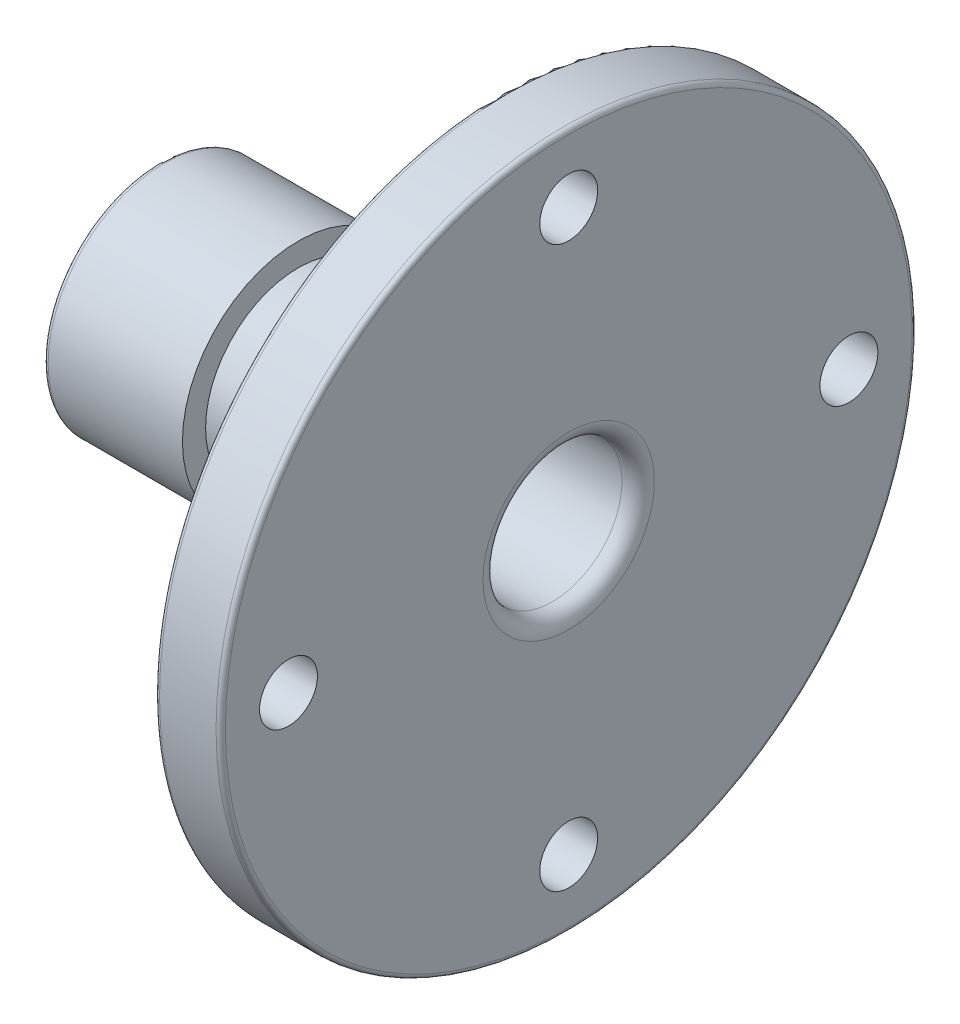
ISO-10303-21;
HEADER;
FILE_DESCRIPTION(('STEP AP214'),'2;1');
FILE_NAME('part.step','',(''),(''),'','','');
FILE_SCHEMA(('AUTOMOTIVE_DESIGN { 1 0 10303 214 1 1 1 1 }'));
ENDSEC;
DATA;
#1=APPLICATION_CONTEXT('core data for automotive mechanical design processes');
#2=APPLICATION_PROTOCOL_DEFINITION('international standard','automotive_design',2000,#1);
#3=PRODUCT_CONTEXT('',#1,'mechanical');
#4=PRODUCT('Part','Part','',(#3));
#5=PRODUCT_RELATED_PRODUCT_CATEGORY('part','',(#4));
#6=PRODUCT_DEFINITION_FORMATION('','',#4);
#7=PRODUCT_DEFINITION_CONTEXT('part definition',#1,'design');
#8=PRODUCT_DEFINITION('design','',#6,#7);
#9=PRODUCT_DEFINITION_SHAPE('','',#8);
#10=(LENGTH_UNIT() NAMED_UNIT(*) SI_UNIT(.MILLI.,.METRE.));
#11=(NAMED_UNIT(*) PLANE_ANGLE_UNIT() SI_UNIT($,.RADIAN.));
#12=(NAMED_UNIT(*) SI_UNIT($,.STERADIAN.) SOLID_ANGLE_UNIT());
#13=UNCERTAINTY_MEASURE_WITH_UNIT(LENGTH_MEASURE(1.E-05),#10,'distance_accuracy_value','');
#14=(GEOMETRIC_REPRESENTATION_CONTEXT(3) GLOBAL_UNCERTAINTY_ASSIGNED_CONTEXT((#13)) GLOBAL_UNIT_ASSIGNED_CONTEXT((#10,
#11,#12)) REPRESENTATION_CONTEXT('',''));
#15=CARTESIAN_POINT('',(0.,0.,0.));
#16=DIRECTION('',(0.,0.,1.));
#17=DIRECTION('',(1.,0.,0.));
#18=AXIS2_PLACEMENT_3D('',#15,#16,#17);
#19=CARTESIAN_POINT('',(0.,20.,0.));
#20=DIRECTION('',(1.,0.,0.));
#21=DIRECTION('',(0.,0.,-1.));
#22=AXIS2_PLACEMENT_3D('',#19,#20,#21);
#23=PLANE('',#22);
#24=CARTESIAN_POINT('',(0.,0.,0.));
#25=DIRECTION('',(1.,0.,0.));
#26=DIRECTION('',(0.,0.,-1.));
#27=AXIS2_PLACEMENT_3D('',#24,#25,#26);
#28=CIRCLE('',#27,24.);
#29=CARTESIAN_POINT('',(0.,0.,-24.));
#30=VERTEX_POINT('',#29);
#31=EDGE_CURVE('E42',#30,#30,#28,.F.);
#32=ORIENTED_EDGE('',*,*,#31,.T.);
#33=EDGE_LOOP('',(#32));
#34=FACE_BOUND('',#33,.T.);
#35=CARTESIAN_POINT('',(0.,0.,0.));
#36=DIRECTION('',(-1.,0.,0.));
#37=DIRECTION('',(0.,0.,1.));
#38=AXIS2_PLACEMENT_3D('',#35,#36,#37);
#39=CIRCLE('',#38,20.);
#40=CARTESIAN_POINT('',(0.,0.,20.));
#41=VERTEX_POINT('',#40);
#42=EDGE_CURVE('E78',#41,#41,#39,.T.);
#43=ORIENTED_EDGE('',*,*,#42,.F.);
#44=EDGE_LOOP('',(#43));
#45=FACE_BOUND('',#44,.T.);
#46=ADVANCED_FACE('F40',(#34,#45),#23,.F.);
#47=CARTESIAN_POINT('',(-1000.,0.,0.));
#48=DIRECTION('',(-1.,0.,0.));
#49=DIRECTION('',(0.,0.,1.));
#50=AXIS2_PLACEMENT_3D('',#47,#48,#49);
#51=CYLINDRICAL_SURFACE('',#50,25.);
#52=CARTESIAN_POINT('',(0.99999999999989,0.,0.));
#53=DIRECTION('',(1.,0.,0.));
#54=DIRECTION('',(0.,0.,-1.));
#55=AXIS2_PLACEMENT_3D('',#52,#53,#54);
#56=CIRCLE('',#55,25.);
#57=CARTESIAN_POINT('',(0.99999999999989,0.,-25.));
#58=VERTEX_POINT('',#57);
#59=EDGE_CURVE('E10',#58,#58,#56,.T.);
#60=ORIENTED_EDGE('',*,*,#59,.T.);
#61=EDGE_LOOP('',(#60));
#62=FACE_BOUND('',#61,.T.);
#63=CARTESIAN_POINT('',(30.,0.,0.));
#64=DIRECTION('',(-1.,0.,0.));
#65=DIRECTION('',(0.,0.,1.));
#66=AXIS2_PLACEMENT_3D('',#63,#64,#65);
#67=CIRCLE('',#66,25.);
#68=CARTESIAN_POINT('',(30.,0.,25.));
#69=VERTEX_POINT('',#68);
#70=EDGE_CURVE('E73',#69,#69,#67,.T.);
#71=ORIENTED_EDGE('',*,*,#70,.T.);
#72=EDGE_LOOP('',(#71));
#73=FACE_BOUND('',#72,.T.);
#74=ADVANCED_FACE('F156',(#62,#73),#51,.T.);
#75=CARTESIAN_POINT('',(30.,25.,0.));
#76=DIRECTION('',(-1.,0.,0.));
#77=DIRECTION('',(0.,0.,1.));
#78=AXIS2_PLACEMENT_3D('',#75,#76,#77);
#79=PLANE('',#78);
#80=ORIENTED_EDGE('',*,*,#70,.F.);
#81=EDGE_LOOP('',(#80));
#82=FACE_BOUND('',#81,.T.);
#83=CARTESIAN_POINT('',(30.,0.,0.));
#84=DIRECTION('',(-1.,0.,0.));
#85=DIRECTION('',(0.,0.,1.));
#86=AXIS2_PLACEMENT_3D('',#83,#84,#85);
#87=CIRCLE('',#86,20.);
#88=CARTESIAN_POINT('',(30.,0.,20.));
#89=VERTEX_POINT('',#88);
#90=EDGE_CURVE('E95',#89,#89,#87,.T.);
#91=ORIENTED_EDGE('',*,*,#90,.T.);
#92=EDGE_LOOP('',(#91));
#93=FACE_BOUND('',#92,.T.);
#94=ADVANCED_FACE('F165',(#82,#93),#79,.F.);
#95=CARTESIAN_POINT('',(-1000.,0.,0.));
#96=DIRECTION('',(-1.,0.,0.));
#97=DIRECTION('',(0.,0.,1.));
#98=AXIS2_PLACEMENT_3D('',#95,#96,#97);
#99=CYLINDRICAL_SURFACE('',#98,20.);
#100=CARTESIAN_POINT('',(73.1999999999999,0.,0.));
#101=DIRECTION('',(1.,0.,0.));
#102=DIRECTION('',(0.,0.,-1.));
#103=AXIS2_PLACEMENT_3D('',#100,#101,#102);
#104=CIRCLE('',#103,20.);
#105=CARTESIAN_POINT('',(73.1999999999999,0.,-20.));
#106=VERTEX_POINT('',#105);
#107=EDGE_CURVE('E48',#106,#106,#104,.F.);
#108=ORIENTED_EDGE('',*,*,#107,.T.);
#109=EDGE_LOOP('',(#108));
#110=FACE_BOUND('',#109,.T.);
#111=ORIENTED_EDGE('',*,*,#90,.F.);
#112=EDGE_LOOP('',(#111));
#113=FACE_BOUND('',#112,.T.);
#114=ADVANCED_FACE('F121',(#110,#113),#99,.T.);
#115=CARTESIAN_POINT('',(74.2,20.,0.));
#116=DIRECTION('',(1.,0.,0.));
#117=DIRECTION('',(0.,0.,-1.));
#118=AXIS2_PLACEMENT_3D('',#115,#116,#117);
#119=PLANE('',#118);
#120=CARTESIAN_POINT('',(74.2,0.,0.));
#121=DIRECTION('',(1.,0.,0.));
#122=DIRECTION('',(0.,0.,-1.));
#123=AXIS2_PLACEMENT_3D('',#120,#121,#122);
#124=CIRCLE('',#123,74.148420880377);
#125=CARTESIAN_POINT('',(74.2,0.,-74.148420880377));
#126=VERTEX_POINT('',#125);
#127=EDGE_CURVE('E55',#126,#126,#124,.F.);
#128=ORIENTED_EDGE('',*,*,#127,.T.);
#129=EDGE_LOOP('',(#128));
#130=FACE_BOUND('',#129,.T.);
#131=CARTESIAN_POINT('',(74.2,0.,0.));
#132=DIRECTION('',(1.,0.,0.));
#133=DIRECTION('',(0.,0.,-1.));
#134=AXIS2_PLACEMENT_3D('',#131,#132,#133);
#135=CIRCLE('',#134,21.);
#136=CARTESIAN_POINT('',(74.2,0.,-21.));
#137=VERTEX_POINT('',#136);
#138=EDGE_CURVE('E60',#137,#137,#135,.T.);
#139=ORIENTED_EDGE('',*,*,#138,.T.);
#140=EDGE_LOOP('',(#139));
#141=FACE_BOUND('',#140,.T.);
#142=CARTESIAN_POINT('',(74.2,60.5,0.));
#143=DIRECTION('',(-1.,0.,0.));
#144=DIRECTION('',(0.,0.,1.));
#145=AXIS2_PLACEMENT_3D('',#142,#143,#144);
#146=CIRCLE('',#145,6.25);
#147=CARTESIAN_POINT('',(74.2,60.5,6.25));
#148=VERTEX_POINT('',#147);
#149=EDGE_CURVE('E90',#148,#148,#146,.T.);
#150=ORIENTED_EDGE('',*,*,#149,.F.);
#151=EDGE_LOOP('',(#150));
#152=FACE_BOUND('',#151,.T.);
#153=CARTESIAN_POINT('',(74.2,0.,-60.5));
#154=DIRECTION('',(-1.,0.,0.));
#155=DIRECTION('',(0.,0.,1.));
#156=AXIS2_PLACEMENT_3D('',#153,#154,#155);
#157=CIRCLE('',#156,6.25);
#158=CARTESIAN_POINT('',(74.2,0.,-54.25));
#159=VERTEX_POINT('',#158);
#160=EDGE_CURVE('E108',#159,#159,#157,.T.);
#161=ORIENTED_EDGE('',*,*,#160,.F.);
#162=EDGE_LOOP('',(#161));
#163=FACE_BOUND('',#162,.T.);
#164=CARTESIAN_POINT('',(74.2,-60.5,0.));
#165=DIRECTION('',(-1.,0.,0.));
#166=DIRECTION('',(0.,0.,-1.));
#167=AXIS2_PLACEMENT_3D('',#164,#165,#166);
#168=CIRCLE('',#167,6.25);
#169=CARTESIAN_POINT('',(74.2,-60.5,-6.24999999999998));
#170=VERTEX_POINT('',#169);
#171=EDGE_CURVE('E106',#170,#170,#168,.T.);
#172=ORIENTED_EDGE('',*,*,#171,.F.);
#173=EDGE_LOOP('',(#172));
#174=FACE_BOUND('',#173,.T.);
#175=CARTESIAN_POINT('',(74.2,4.44089209850063E-13,60.5));
#176=DIRECTION('',(-1.,0.,0.));
#177=DIRECTION('',(0.,0.,-1.));
#178=AXIS2_PLACEMENT_3D('',#175,#176,#177);
#179=CIRCLE('',#178,6.25000000000001);
#180=CARTESIAN_POINT('',(74.2,4.44089209850063E-13,54.25));
#181=VERTEX_POINT('',#180);
#182=EDGE_CURVE('E103',#181,#181,#179,.T.);
#183=ORIENTED_EDGE('',*,*,#182,.F.);
#184=EDGE_LOOP('',(#183));
#185=FACE_BOUND('',#184,.T.);
#186=ADVANCED_FACE('F117',(#130,#141,#152,#163,#174,#185),#119,.F.);
#187=CARTESIAN_POINT('',(-1000.,0.,0.));
#188=DIRECTION('',(-1.,0.,0.));
#189=DIRECTION('',(0.,0.,1.));
#190=AXIS2_PLACEMENT_3D('',#187,#188,#189);
#191=CYLINDRICAL_SURFACE('',#190,75.148420880377);
#192=CARTESIAN_POINT('',(87.3999999999999,0.,0.));
#193=DIRECTION('',(-1.,0.,0.));
#194=DIRECTION('',(0.,0.,1.));
#195=AXIS2_PLACEMENT_3D('',#192,#193,#194);
#196=CIRCLE('',#195,75.148420880377);
#197=CARTESIAN_POINT('',(87.3999999999999,0.,75.148420880377));
#198=VERTEX_POINT('',#197);
#199=EDGE_CURVE('E62',#198,#198,#196,.T.);
#200=ORIENTED_EDGE('',*,*,#199,.T.);
#201=EDGE_LOOP('',(#200));
#202=FACE_BOUND('',#201,.T.);
#203=CARTESIAN_POINT('',(75.1999999999999,0.,0.));
#204=DIRECTION('',(1.,0.,0.));
#205=DIRECTION('',(0.,0.,-1.));
#206=AXIS2_PLACEMENT_3D('',#203,#204,#205);
#207=CIRCLE('',#206,75.148420880377);
#208=CARTESIAN_POINT('',(75.1999999999999,0.,-75.148420880377));
#209=VERTEX_POINT('',#208);
#210=EDGE_CURVE('E69',#209,#209,#207,.T.);
#211=ORIENTED_EDGE('',*,*,#210,.T.);
#212=EDGE_LOOP('',(#211));
#213=FACE_BOUND('',#212,.T.);
#214=ADVANCED_FACE('F124',(#202,#213),#191,.T.);
#215=CARTESIAN_POINT('',(88.4,75.148420880377,0.));
#216=DIRECTION('',(-1.,0.,0.));
#217=DIRECTION('',(0.,0.,1.));
#218=AXIS2_PLACEMENT_3D('',#215,#216,#217);
#219=PLANE('',#218);
#220=CARTESIAN_POINT('',(88.4,0.,0.));
#221=DIRECTION('',(-1.,0.,0.));
#222=DIRECTION('',(0.,0.,1.));
#223=AXIS2_PLACEMENT_3D('',#220,#221,#222);
#224=CIRCLE('',#223,74.148420880377);
#225=CARTESIAN_POINT('',(88.4,0.,74.148420880377));
#226=VERTEX_POINT('',#225);
#227=EDGE_CURVE('E58',#226,#226,#224,.F.);
#228=ORIENTED_EDGE('',*,*,#227,.T.);
#229=EDGE_LOOP('',(#228));
#230=FACE_BOUND('',#229,.T.);
#231=CARTESIAN_POINT('',(88.4,0.,0.));
#232=DIRECTION('',(-1.,0.,0.));
#233=DIRECTION('',(0.,0.,1.));
#234=AXIS2_PLACEMENT_3D('',#231,#232,#233);
#235=CIRCLE('',#234,18.5);
#236=CARTESIAN_POINT('',(88.4,0.,18.5));
#237=VERTEX_POINT('',#236);
#238=EDGE_CURVE('E75',#237,#237,#235,.T.);
#239=ORIENTED_EDGE('',*,*,#238,.T.);
#240=EDGE_LOOP('',(#239));
#241=FACE_BOUND('',#240,.T.);
#242=CARTESIAN_POINT('',(88.4,60.5,0.));
#243=DIRECTION('',(-1.,0.,0.));
#244=DIRECTION('',(0.,0.,1.));
#245=AXIS2_PLACEMENT_3D('',#242,#243,#244);
#246=CIRCLE('',#245,6.25);
#247=CARTESIAN_POINT('',(88.4,60.5,6.25));
#248=VERTEX_POINT('',#247);
#249=EDGE_CURVE('E76',#248,#248,#246,.T.);
#250=ORIENTED_EDGE('',*,*,#249,.T.);
#251=EDGE_LOOP('',(#250));
#252=FACE_BOUND('',#251,.T.);
#253=CARTESIAN_POINT('',(88.4,0.,-60.5));
#254=DIRECTION('',(-1.,0.,0.));
#255=DIRECTION('',(0.,0.,1.));
#256=AXIS2_PLACEMENT_3D('',#253,#254,#255);
#257=CIRCLE('',#256,6.25);
#258=CARTESIAN_POINT('',(88.4,0.,-54.25));
#259=VERTEX_POINT('',#258);
#260=EDGE_CURVE('E79',#259,#259,#257,.T.);
#261=ORIENTED_EDGE('',*,*,#260,.T.);
#262=EDGE_LOOP('',(#261));
#263=FACE_BOUND('',#262,.T.);
#264=CARTESIAN_POINT('',(88.4,-60.5,0.));
#265=DIRECTION('',(-1.,0.,0.));
#266=DIRECTION('',(0.,0.,1.));
#267=AXIS2_PLACEMENT_3D('',#264,#265,#266);
#268=CIRCLE('',#267,6.25);
#269=CARTESIAN_POINT('',(88.4,-60.5,6.25000000000003));
#270=VERTEX_POINT('',#269);
#271=EDGE_CURVE('E85',#270,#270,#268,.T.);
#272=ORIENTED_EDGE('',*,*,#271,.T.);
#273=EDGE_LOOP('',(#272));
#274=FACE_BOUND('',#273,.T.);
#275=CARTESIAN_POINT('',(88.4,4.44089209850063E-13,60.5));
#276=DIRECTION('',(-1.,0.,0.));
#277=DIRECTION('',(0.,0.,1.));
#278=AXIS2_PLACEMENT_3D('',#275,#276,#277);
#279=CIRCLE('',#278,6.25000000000001);
#280=CARTESIAN_POINT('',(88.4,4.44089209850063E-13,66.75));
#281=VERTEX_POINT('',#280);
#282=EDGE_CURVE('E88',#281,#281,#279,.T.);
#283=ORIENTED_EDGE('',*,*,#282,.T.);
#284=EDGE_LOOP('',(#283));
#285=FACE_BOUND('',#284,.T.);
#286=ADVANCED_FACE('F138',(#230,#241,#252,#263,#274,#285),#219,.F.);
#287=CARTESIAN_POINT('',(-1000.,0.,0.));
#288=DIRECTION('',(-1.,0.,0.));
#289=DIRECTION('',(0.,0.,1.));
#290=AXIS2_PLACEMENT_3D('',#287,#288,#289);
#291=CYLINDRICAL_SURFACE('',#290,15.);
#292=CARTESIAN_POINT('',(84.9,0.,0.));
#293=DIRECTION('',(-1.,0.,0.));
#294=DIRECTION('',(0.,0.,1.));
#295=AXIS2_PLACEMENT_3D('',#292,#293,#294);
#296=CIRCLE('',#295,15.);
#297=CARTESIAN_POINT('',(84.9,0.,15.));
#298=VERTEX_POINT('',#297);
#299=EDGE_CURVE('E68',#298,#298,#296,.F.);
#300=ORIENTED_EDGE('',*,*,#299,.T.);
#301=EDGE_LOOP('',(#300));
#302=FACE_BOUND('',#301,.T.);
#303=CARTESIAN_POINT('',(24.,0.,0.));
#304=DIRECTION('',(-1.,0.,0.));
#305=DIRECTION('',(0.,0.,1.));
#306=AXIS2_PLACEMENT_3D('',#303,#304,#305);
#307=CIRCLE('',#306,15.);
#308=CARTESIAN_POINT('',(24.,0.,15.));
#309=VERTEX_POINT('',#308);
#310=EDGE_CURVE('E92',#309,#309,#307,.T.);
#311=ORIENTED_EDGE('',*,*,#310,.T.);
#312=EDGE_LOOP('',(#311));
#313=FACE_BOUND('',#312,.T.);
#314=ADVANCED_FACE('F143',(#302,#313),#291,.F.);
#315=CARTESIAN_POINT('',(24.,15.,0.));
#316=DIRECTION('',(1.,0.,0.));
#317=DIRECTION('',(0.,0.,-1.));
#318=AXIS2_PLACEMENT_3D('',#315,#316,#317);
#319=PLANE('',#318);
#320=ORIENTED_EDGE('',*,*,#310,.F.);
#321=EDGE_LOOP('',(#320));
#322=FACE_BOUND('',#321,.T.);
#323=CARTESIAN_POINT('',(24.,0.,0.));
#324=DIRECTION('',(-1.,0.,0.));
#325=DIRECTION('',(0.,0.,1.));
#326=AXIS2_PLACEMENT_3D('',#323,#324,#325);
#327=CIRCLE('',#326,20.);
#328=CARTESIAN_POINT('',(24.,0.,20.));
#329=VERTEX_POINT('',#328);
#330=EDGE_CURVE('E98',#329,#329,#327,.T.);
#331=ORIENTED_EDGE('',*,*,#330,.T.);
#332=EDGE_LOOP('',(#331));
#333=FACE_BOUND('',#332,.T.);
#334=ADVANCED_FACE('F149',(#322,#333),#319,.F.);
#335=CARTESIAN_POINT('',(-1000.,0.,0.));
#336=DIRECTION('',(-1.,0.,0.));
#337=DIRECTION('',(0.,0.,1.));
#338=AXIS2_PLACEMENT_3D('',#335,#336,#337);
#339=CYLINDRICAL_SURFACE('',#338,20.);
#340=ORIENTED_EDGE('',*,*,#330,.F.);
#341=EDGE_LOOP('',(#340));
#342=FACE_BOUND('',#341,.T.);
#343=ORIENTED_EDGE('',*,*,#42,.T.);
#344=EDGE_LOOP('',(#343));
#345=FACE_BOUND('',#344,.T.);
#346=ADVANCED_FACE('F134',(#342,#345),#339,.F.);
#347=CARTESIAN_POINT('',(126.2,4.44089209850063E-13,60.5));
#348=DIRECTION('',(-1.,0.,0.));
#349=DIRECTION('',(0.,0.,1.));
#350=AXIS2_PLACEMENT_3D('',#347,#348,#349);
#351=CYLINDRICAL_SURFACE('',#350,6.25000000000001);
#352=ORIENTED_EDGE('',*,*,#182,.T.);
#353=EDGE_LOOP('',(#352));
#354=FACE_BOUND('',#353,.T.);
#355=ORIENTED_EDGE('',*,*,#282,.F.);
#356=EDGE_LOOP('',(#355));
#357=FACE_BOUND('',#356,.T.);
#358=ADVANCED_FACE('F131',(#354,#357),#351,.F.);
#359=CARTESIAN_POINT('',(126.2,-60.5,0.));
#360=DIRECTION('',(-1.,0.,0.));
#361=DIRECTION('',(0.,0.,1.));
#362=AXIS2_PLACEMENT_3D('',#359,#360,#361);
#363=CYLINDRICAL_SURFACE('',#362,6.25);
#364=ORIENTED_EDGE('',*,*,#171,.T.);
#365=EDGE_LOOP('',(#364));
#366=FACE_BOUND('',#365,.T.);
#367=ORIENTED_EDGE('',*,*,#271,.F.);
#368=EDGE_LOOP('',(#367));
#369=FACE_BOUND('',#368,.T.);
#370=ADVANCED_FACE('F133',(#366,#369),#363,.F.);
#371=CARTESIAN_POINT('',(126.2,0.,-60.5));
#372=DIRECTION('',(-1.,0.,0.));
#373=DIRECTION('',(0.,0.,1.));
#374=AXIS2_PLACEMENT_3D('',#371,#372,#373);
#375=CYLINDRICAL_SURFACE('',#374,6.25);
#376=ORIENTED_EDGE('',*,*,#160,.T.);
#377=EDGE_LOOP('',(#376));
#378=FACE_BOUND('',#377,.T.);
#379=ORIENTED_EDGE('',*,*,#260,.F.);
#380=EDGE_LOOP('',(#379));
#381=FACE_BOUND('',#380,.T.);
#382=ADVANCED_FACE('F228',(#378,#381),#375,.F.);
#383=CARTESIAN_POINT('',(126.2,60.5,0.));
#384=DIRECTION('',(-1.,0.,0.));
#385=DIRECTION('',(0.,0.,1.));
#386=AXIS2_PLACEMENT_3D('',#383,#384,#385);
#387=CYLINDRICAL_SURFACE('',#386,6.25);
#388=ORIENTED_EDGE('',*,*,#149,.T.);
#389=EDGE_LOOP('',(#388));
#390=FACE_BOUND('',#389,.T.);
#391=ORIENTED_EDGE('',*,*,#249,.F.);
#392=EDGE_LOOP('',(#391));
#393=FACE_BOUND('',#392,.T.);
#394=ADVANCED_FACE('F113',(#390,#393),#387,.F.);
#395=CARTESIAN_POINT('',(84.9,0.,0.));
#396=DIRECTION('',(-1.,0.,0.));
#397=DIRECTION('',(0.,0.,1.));
#398=AXIS2_PLACEMENT_3D('',#395,#396,#397);
#399=TOROIDAL_SURFACE('',#398,18.5,3.5);
#400=ORIENTED_EDGE('',*,*,#299,.F.);
#401=EDGE_LOOP('',(#400));
#402=FACE_BOUND('',#401,.T.);
#403=ORIENTED_EDGE('',*,*,#238,.F.);
#404=EDGE_LOOP('',(#403));
#405=FACE_BOUND('',#404,.T.);
#406=ADVANCED_FACE('F170',(#402,#405),#399,.T.);
#407=CARTESIAN_POINT('',(87.3999999999999,0.,0.));
#408=DIRECTION('',(-1.,0.,0.));
#409=DIRECTION('',(0.,0.,1.));
#410=AXIS2_PLACEMENT_3D('',#407,#408,#409);
#411=TOROIDAL_SURFACE('',#410,74.148420880377,1.);
#412=ORIENTED_EDGE('',*,*,#227,.F.);
#413=EDGE_LOOP('',(#412));
#414=FACE_BOUND('',#413,.T.);
#415=ORIENTED_EDGE('',*,*,#199,.F.);
#416=EDGE_LOOP('',(#415));
#417=FACE_BOUND('',#416,.T.);
#418=ADVANCED_FACE('F166',(#414,#417),#411,.T.);
#419=CARTESIAN_POINT('',(75.1999999999999,0.,0.));
#420=DIRECTION('',(1.,0.,0.));
#421=DIRECTION('',(0.,0.,-1.));
#422=AXIS2_PLACEMENT_3D('',#419,#420,#421);
#423=TOROIDAL_SURFACE('',#422,74.148420880377,1.);
#424=ORIENTED_EDGE('',*,*,#210,.F.);
#425=EDGE_LOOP('',(#424));
#426=FACE_BOUND('',#425,.T.);
#427=ORIENTED_EDGE('',*,*,#127,.F.);
#428=EDGE_LOOP('',(#427));
#429=FACE_BOUND('',#428,.T.);
#430=ADVANCED_FACE('F175',(#426,#429),#423,.T.);
#431=CARTESIAN_POINT('',(73.1999999999999,0.,0.));
#432=DIRECTION('',(1.,0.,0.));
#433=DIRECTION('',(0.,0.,-1.));
#434=AXIS2_PLACEMENT_3D('',#431,#432,#433);
#435=TOROIDAL_SURFACE('',#434,21.,1.);
#436=ORIENTED_EDGE('',*,*,#138,.F.);
#437=EDGE_LOOP('',(#436));
#438=FACE_BOUND('',#437,.T.);
#439=ORIENTED_EDGE('',*,*,#107,.F.);
#440=EDGE_LOOP('',(#439));
#441=FACE_BOUND('',#440,.T.);
#442=ADVANCED_FACE('F174',(#438,#441),#435,.F.);
#443=CARTESIAN_POINT('',(0.99999999999989,0.,0.));
#444=DIRECTION('',(1.,0.,0.));
#445=DIRECTION('',(0.,0.,-1.));
#446=AXIS2_PLACEMENT_3D('',#443,#444,#445);
#447=TOROIDAL_SURFACE('',#446,24.,1.);
#448=ORIENTED_EDGE('',*,*,#59,.F.);
#449=EDGE_LOOP('',(#448));
#450=FACE_BOUND('',#449,.T.);
#451=ORIENTED_EDGE('',*,*,#31,.F.);
#452=EDGE_LOOP('',(#451));
#453=FACE_BOUND('',#452,.T.);
#454=ADVANCED_FACE('F39',(#450,#453),#447,.T.);
#455=CLOSED_SHELL('',(#46,#74,#94,#114,#186,#214,#286,#314,#334,#346,#358,#370,#382,#394,#406,
#418,#430,#442,#454));
#456=MANIFOLD_SOLID_BREP('B2',#455);
#457=ADVANCED_BREP_SHAPE_REPRESENTATION('',(#18,#456),#14);
#458=SHAPE_DEFINITION_REPRESENTATION(#9,#457);
ENDSEC;
END-ISO-10303-21;
